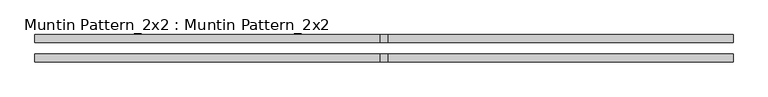
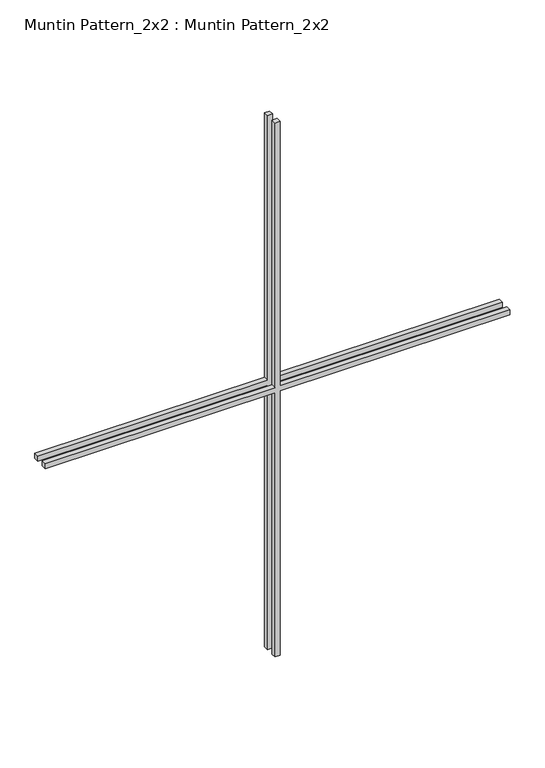
"""IFC4 building model written with IfcOpenShell, lengths in millimetres: proxy geometry, Muntin Pattern_2x2 : Muntin Pattern_2x2."""

from ifc_helpers import new_model, si_unit, frame, origin, place, context, project, spatial, polyline, outline, extrude, source, transform, mapped, element, save


def muntin_pattern_2x2_muntin_pattern_2x2_511ed329(model_context):
    return source(origin(), model_context, "Body", "SweptSolid", [
        extrude(outline(polyline([(698.5, -6.35), (698.5, -570.0914087), (685.8, -570.0914087), (685.8, -6.35), (0.0, -6.35), (0.0, 6.35), (685.8, 6.35), (685.8, 570.0914087), (698.5, 570.0914087), (698.5, 6.35), (1384.3, 6.35), (1384.3, -6.35), (698.5, -6.35)])), frame((0.0, 9.525, 0.0), z_axis=(0.0, 1.0, 0.0), x_axis=(0.0, 0.0, 1.0)), (0.0, 0.0, 1.0), 12.7),
        extrude(outline(polyline([(698.5, -6.35), (698.5, -570.0914087), (685.8, -570.0914087), (685.8, -6.35), (0.0, -6.35), (0.0, 6.35), (685.8, 6.35), (685.8, 570.0914087), (698.5, 570.0914087), (698.5, 6.35), (1384.3, 6.35), (1384.3, -6.35), (698.5, -6.35)])), frame((0.0, -22.225, 0.0), z_axis=(0.0, 1.0, 0.0), x_axis=(0.0, 0.0, 1.0)), (0.0, 0.0, 1.0), 12.7),
    ])


if __name__ == "__main__":
    model = new_model("IFC4")
    model_context = context("Model", 3, world=origin())
    ifc_project = project(units=[si_unit("LENGTHUNIT", "METRE", prefix="MILLI")], contexts=[model_context])
    site = spatial("IfcSite", under=ifc_project)
    building = spatial("IfcBuilding", under=site)
    placement = place(None, origin())
    muntin_pattern_2x2_muntin_pattern_2x2_shape = muntin_pattern_2x2_muntin_pattern_2x2_511ed329(model_context)
    element("IfcBuildingElementProxy", 1, Name="Muntin Pattern_2x2 : Muntin Pattern_2x2", ObjectType="Muntin Pattern_2x2 : Muntin Pattern_2x2", at=placement, inside=building, context=model_context, shape_type="MappedRepresentation", body=[
        mapped(muntin_pattern_2x2_muntin_pattern_2x2_shape, transform((0.0, 0.0, 0.0), x_axis=(1.0, 0.0, 0.0), y_axis=(0.0, 1.0, 0.0), z_axis=(0.0, 0.0, 1.0))),
    ])
    save(model, "model.ifc")

# Revit data of these elements
# Type "Muntin Pattern_2x2 : Muntin Pattern_2x2"
#   Width [instance default] = 4' - 0"
#   Thickness = 0' - 0 1/2"
#   Height [instance default] = 4' - 0"
#   Distance = 0' - 0 3/4"
#   Interior Material [instance default] = none
#   Exterior Material [instance default] = none
#   Default Elevation = 0
# Element 1 (IfcBuildingElementProxy, "Muntin Pattern_2x2 : Muntin Pattern_2x2")
#   Width = 3' - 8.88909"
#   Height = 4' - 6 1/2"
#   Interior Material = Wood - Stained
#   Exterior Material = Clad - White
#   Materials on its faces: "Clad - White", "Wood - Stained"
# Materials
#   "Clad - White": class "Wood", colour RGB 242 242 238, transparency 0, Cost = 0
#   "Wood - Stained": class "Wood", colour RGB 227 170 128, transparency 0, Cost = 0
